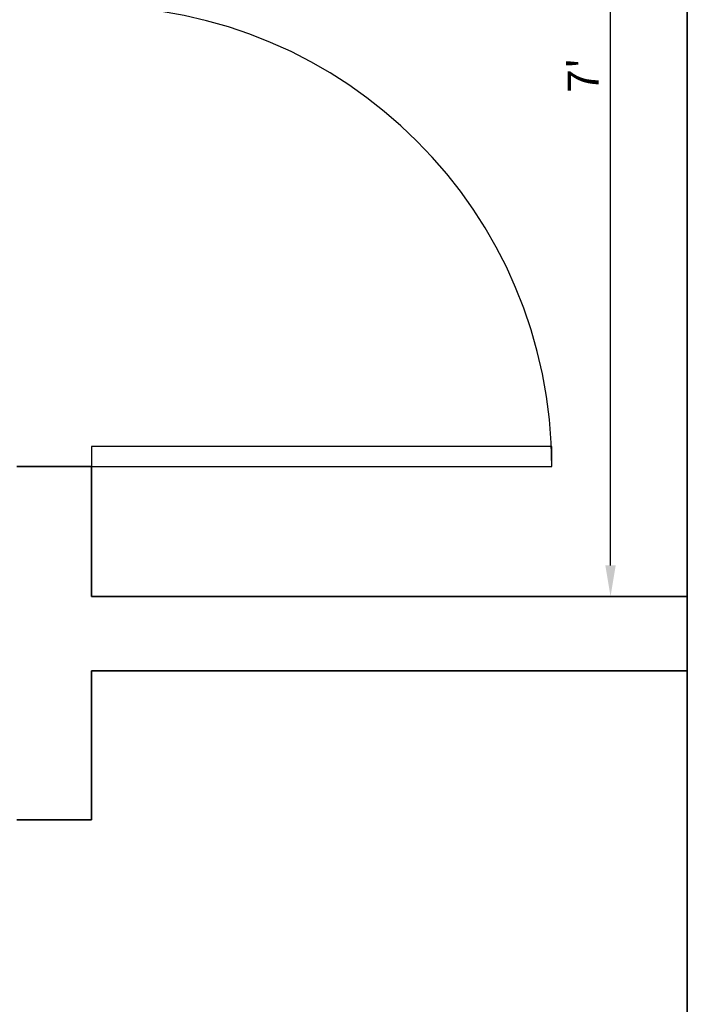
# Model space of a CAD drawing. Units: inches. Extents: x 2025 to 2528, y 1525 to 2336.
# Tile 15 of 18: x 2255 to 2309, y 2167 to 2246. Entities that reach past the tile are written whole.
import ezdxf

# ---------------------------------------------------------------- set-up
doc = ezdxf.new("R2010")
doc.units = ezdxf.units.IN
for name, color, linetype, lineweight in [('A-ANNO-DIMS', 2, 'Continuous', 18), ('A-DOOR', 3, 'Continuous', 25), ('A-WALL', 7, 'Continuous', 35)]:
    doc.layers.add(name, color=color, linetype=linetype, lineweight=lineweight)
doc.styles.get("Standard").update_dxf_attribs({"font": 'arial.ttf'})
doc.dimstyles.new('Copy of ISO-25', dxfattribs={"dimtxt": 2.5, "dimasz": 2.5, "dimexe": 1.25, "dimexo": 0.625, "dimtad": 1, "dimdec": 1, "dimlunit": 4, "dimtxsty": 'Standard', "dimcen": 2.5, "dimadec": 0, "dimazin": 0, "dimtfac": 1, "dimtdec": 1, "dimtmove": 0, "dimatfit": 3, "dimfxl": 1, "dimarcsym": 0})

# ---------------------------------------------------------------- blocks, each defined once
blk = doc.blocks.new('*U2')
for p, q in [((0, 0), (0, 6)), ((40, 0), (40, 6))]:
    blk.add_line(p, q)
blk.add_lwpolyline([(0, 0), (0, -40), (1.75, -40), (1.75, 0)], close=True)
blk.add_arc((0, 0), 40, 270, 0)
blk = doc.blocks.new('*D9')
at = {"layer": 'A-ANNO-DIMS', "color": 0, "lineweight": -2, "transparency": 16777216}
for p, q in [((2308.388, 2283.412), (2301.577, 2283.412)), ((2302.827, 2201.912), (2302.827, 2280.912)), ((2308.388, 2199.412), (2301.577, 2199.412))]:
    blk.add_line(p, q, dxfattribs=at)
at = {"layer": 'A-ANNO-DIMS', "color": 0, "transparency": 16777216}
for points in [[(2302.41, 2280.912), (2303.243, 2280.912), (2302.827, 2283.412)], [(2302.41, 2201.912), (2303.243, 2201.912), (2302.827, 2199.412)]]:
    blk.add_solid(points, dxfattribs=at)
at = {"layer": 'Defpoints', "color": 0, "transparency": 16777216}
for p in [(2302.827, 2283.412), (2309.013, 2283.412), (2309.013, 2199.412)]:
    blk.add_point(p, dxfattribs=at)
at = {"layer": 'A-ANNO-DIMS', "color": 0, "transparency": 16777216, "insert": (2300.952, 2241.412), "char_height": 2.5, "attachment_point": 5, "rotation": 90}
blk.add_mtext("7'", dxfattribs=at)
blk = doc.blocks.new('*D80')
at = {"layer": 'A-ANNO-DIMS', "color": 0, "lineweight": -2, "transparency": 16777216}
for p, q in [((2065.388, 2292.412), (2027.213, 2292.412)), ((2028.463, 1566.912), (2028.463, 2289.912)), ((2285.388, 1564.412), (2027.213, 1564.412))]:
    blk.add_line(p, q, dxfattribs=at)
at = {"layer": 'A-ANNO-DIMS', "color": 0, "transparency": 16777216}
for points in [[(2028.046, 2289.912), (2028.88, 2289.912), (2028.463, 2292.412)], [(2028.046, 1566.912), (2028.88, 1566.912), (2028.463, 1564.412)]]:
    blk.add_solid(points, dxfattribs=at)
at = {"layer": 'Defpoints', "color": 0, "transparency": 16777216}
for p in [(2028.463, 2292.412), (2066.013, 2292.412), (2286.013, 1564.412)]:
    blk.add_point(p, dxfattribs=at)
at = {"layer": 'A-ANNO-DIMS', "color": 0, "transparency": 16777216, "insert": (2026.561, 1928.412), "char_height": 2.5, "attachment_point": 5, "rotation": 90}
blk.add_mtext('60\'-8"', dxfattribs=at)

msp = doc.modelspace()

# ---------------------------------------------------------------- linework, layer by layer
at = {"layer": 'A-WALL'}
for p, q in [((2309.013, 2283.412), (2309.013, 2115.412)), ((2309.013, 2283.412), (2309.013, 2199.412)), ((2261.013, 2209.877), (2255.013, 2209.877)), ((2261.013, 2199.412), (2261.013, 2209.877)), ((2309.013, 2199.412), (2261.013, 2199.412)), ((2309.013, 2193.412), (2261.013, 2193.412)), ((2261.013, 2181.412), (2261.013, 2193.412)), ((2255.013, 2181.412), (2261.013, 2181.412))]:
    msp.add_line(p, q, dxfattribs=at)

# ---------------------------------------------------------------- block references
at = {"layer": 'A-DOOR', "xscale": 0.9271117355112991, "yscale": 0.9271117355112991, "zscale": 0.9271117355112991, "rotation": 90}
msp.add_blockref('*U2', (2261.013, 2209.877), dxfattribs=at)

# ---------------------------------------------------------------- dimensions: what is measured, and where the dimension line sits
at = {"layer": 'A-ANNO-DIMS'}
for base, p1, p2, override, picture, middle in [((2028.463, 2292.412), (2286.013, 1564.412), (2066.013, 2292.412), {"dimdec": 1, "dimlfac": 1, "dimrnd": 0, "dimzin": 1, "dimdsep": 46, "dimlunit": 4, "dimfrac": 2}, '*D80', (2026.561, 1928.412)), ((2302.827, 2283.412), (2309.013, 2199.412), (2309.013, 2283.412), {"dimclrd": 0, "dimclre": 0, "dimclrt": 0}, '*D9', (2300.952, 2241.412))]:
    dim = msp.add_linear_dim(base=base, p1=p1, p2=p2, angle=90, dimstyle='Copy of ISO-25', override=override, dxfattribs=at)
    dim.commit()
    dim.dimension.update_dxf_attribs({"geometry": picture, "text_midpoint": middle})

doc.saveas('drawing.dxf')
